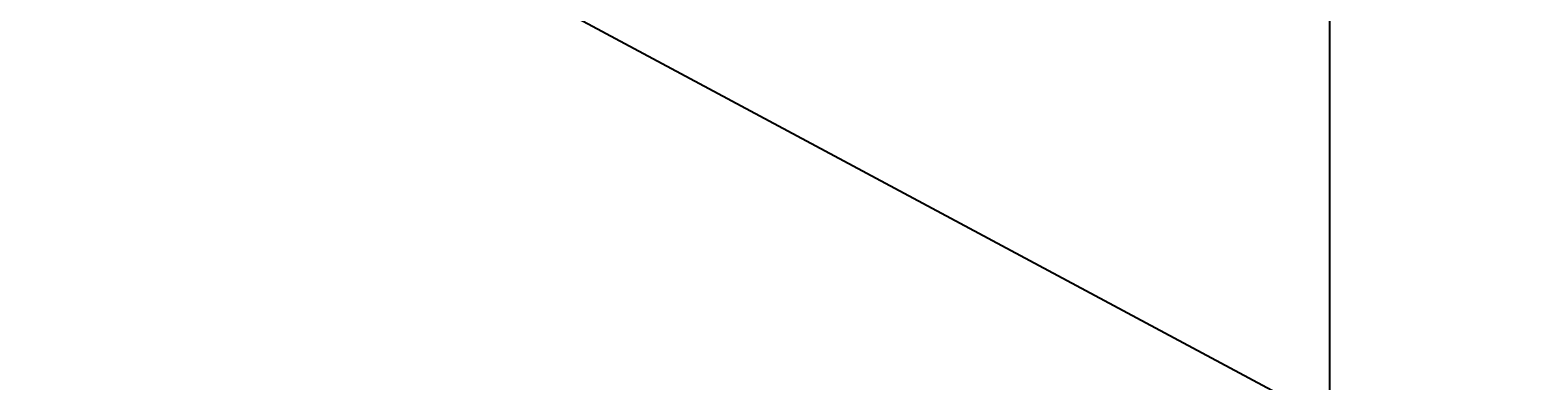
# Model space of a CAD drawing. Units: inches. Extents: x 35362 to 73946, y 43607 to 67532.
# Tile 118 of 134: x 50905 to 51049, y 49061 to 49095. Entities that reach past the tile are written whole.
import ezdxf

# ---------------------------------------------------------------- set-up
doc = ezdxf.new("R2010")
doc.units = ezdxf.units.IN
doc.header["$MEASUREMENT"] = 0
doc.layers.add('A-ANNO-DIMS', color=2, linetype='Continuous', lineweight=18)
doc.layers.add('E-SYMB', color=1, linetype='Continuous', lineweight=25)
doc.styles.get("Standard").update_dxf_attribs({"font": 'arial.ttf'})
doc.dimstyles.get("Standard").update_dxf_attribs({"dimtxt": 0.18, "dimasz": 0.18, "dimexe": 0.18, "dimexo": 0.0625, "dimgap": 0.09, "dimtad": 0, "dimtih": 1, "dimtoh": 1, "dimdec": 4, "dimzin": 0, "dimdsep": 46, "dimtxsty": 'Standard', "dimcen": 0.09, "dimadec": 0, "dimazin": 0, "dimtfac": 1, "dimtdec": 4, "dimtofl": 0, "dimtmove": 0, "dimatfit": 3, "dimfxl": 1, "dimtolj": 1, "dimtzin": 0, "dimarcsym": 0})

# ---------------------------------------------------------------- blocks, each defined once
blk = doc.blocks.new('*D11')
at = {"layer": 'A-ANNO-DIMS', "color": 0, "lineweight": -2, "transparency": 16777216}
for p, q in [((47978.66, 56028.77), (47978.66, 43606.68)), ((53109.76, 56028.77), (53109.76, 43606.68)), ((47978.84, 43606.86), (50543.87, 43606.86)), ((53109.58, 43606.86), (50544.55, 43606.86))]:
    blk.add_line(p, q, dxfattribs=at)
at = {"layer": 'A-ANNO-DIMS', "color": 0, "transparency": 16777216}
for points in [[(47978.84, 43606.89), (47978.84, 43606.83), (47978.66, 43606.86)], [(53109.58, 43606.89), (53109.58, 43606.83), (53109.76, 43606.86)]]:
    blk.add_solid(points, dxfattribs=at)
at = {"layer": 'Defpoints', "color": 0, "transparency": 16777216}
for p in [(47978.66, 56028.84), (53109.76, 56028.84), (53109.76, 43606.86)]:
    blk.add_point(p, dxfattribs=at)
at = {"layer": 'A-ANNO-DIMS', "color": 0, "transparency": 16777216, "insert": (50544.21, 43606.86), "char_height": 0.18, "attachment_point": 5}
blk.add_mtext('\\A1;5131', dxfattribs=at)
blk = doc.blocks.new('*D13')
at = {"layer": 'A-ANNO-DIMS', "color": 0, "lineweight": -2, "transparency": 16777216}
for p, q in [((48373.49, 51694.02), (48373.49, 43606.68)), ((51029.04, 51694.02), (51029.04, 43606.68)), ((48373.67, 43606.86), (49700.8, 43606.86)), ((51028.86, 43606.86), (49701.73, 43606.86))]:
    blk.add_line(p, q, dxfattribs=at)
at = {"layer": 'A-ANNO-DIMS', "color": 0, "transparency": 16777216}
for points in [[(48373.67, 43606.89), (48373.67, 43606.83), (48373.49, 43606.86)], [(51028.86, 43606.89), (51028.86, 43606.83), (51029.04, 43606.86)]]:
    blk.add_solid(points, dxfattribs=at)
at = {"layer": 'Defpoints', "color": 0, "transparency": 16777216}
for p in [(48373.49, 51694.09), (51029.04, 51694.09), (51029.04, 43606.86)]:
    blk.add_point(p, dxfattribs=at)
at = {"layer": 'A-ANNO-DIMS', "color": 0, "transparency": 16777216, "insert": (49701.27, 43606.86), "char_height": 0.18, "attachment_point": 5}
blk.add_mtext('\\A1;2655.6', dxfattribs=at)
blk = doc.blocks.new('*D17')
at = {"layer": 'A-ANNO-DIMS', "color": 0, "lineweight": -2, "transparency": 16777216}
for p, q in [((49923.31, 61293.22), (49923.31, 43606.68)), ((51913.93, 61293.22), (51913.93, 43606.68)), ((49923.49, 43606.86), (50918.16, 43606.86)), ((51913.75, 43606.86), (50919.07, 43606.86))]:
    blk.add_line(p, q, dxfattribs=at)
at = {"layer": 'A-ANNO-DIMS', "color": 0, "transparency": 16777216}
for points in [[(49923.49, 43606.89), (49923.49, 43606.83), (49923.31, 43606.86)], [(51913.75, 43606.89), (51913.75, 43606.83), (51913.93, 43606.86)]]:
    blk.add_solid(points, dxfattribs=at)
at = {"layer": 'Defpoints', "color": 0, "transparency": 16777216}
for p in [(49923.31, 61293.29), (51913.93, 61293.29), (51913.93, 43606.86)]:
    blk.add_point(p, dxfattribs=at)
at = {"layer": 'A-ANNO-DIMS', "color": 0, "transparency": 16777216, "insert": (50918.62, 43606.86), "char_height": 0.18, "attachment_point": 5}
blk.add_mtext('\\A1;1990.6', dxfattribs=at)
blk = doc.blocks.new('*D67')
at = {"layer": 'A-ANNO-DIMS', "color": 0, "lineweight": -2, "transparency": 16777216}
for p, q in [((56873.54, 53351.53), (35361.77, 53351.53)), ((35361.95, 53351.35), (35361.95, 49400.89)), ((35361.95, 45450.07), (35361.95, 49400.53)), ((53793.58, 45449.89), (35361.77, 45449.89))]:
    blk.add_line(p, q, dxfattribs=at)
at = {"layer": 'A-ANNO-DIMS', "color": 0, "transparency": 16777216}
for points in [[(35361.92, 53351.35), (35361.98, 53351.35), (35361.95, 53351.53)], [(35361.92, 45450.07), (35361.98, 45450.07), (35361.95, 45449.89)]]:
    blk.add_solid(points, dxfattribs=at)
at = {"layer": 'Defpoints', "color": 0, "transparency": 16777216}
for p in [(35361.95, 53351.53), (56873.6, 53351.53), (53793.64, 45449.89)]:
    blk.add_point(p, dxfattribs=at)
at = {"layer": 'A-ANNO-DIMS', "color": 0, "transparency": 16777216, "insert": (35361.95, 49400.71), "char_height": 0.18, "attachment_point": 5}
blk.add_mtext('\\A1;7901.6', dxfattribs=at)
blk = doc.blocks.new('*D84')
at = {"layer": 'A-ANNO-DIMS', "color": 0, "lineweight": -2, "transparency": 16777216}
for p, q in [((55540.23, 49259.94), (35361.77, 49259.94)), ((35361.95, 49259.76), (35361.95, 49115.14)), ((35361.95, 48970.16), (35361.95, 49114.78)), ((55540.23, 48969.98), (35361.77, 48969.98))]:
    blk.add_line(p, q, dxfattribs=at)
at = {"layer": 'A-ANNO-DIMS', "color": 0, "transparency": 16777216}
for points in [[(35361.92, 49259.76), (35361.98, 49259.76), (35361.95, 49259.94)], [(35361.92, 48970.16), (35361.98, 48970.16), (35361.95, 48969.98)]]:
    blk.add_solid(points, dxfattribs=at)
at = {"layer": 'Defpoints', "color": 0, "transparency": 16777216}
for p in [(35361.95, 49259.94), (55540.3, 49259.94), (55540.3, 48969.98)]:
    blk.add_point(p, dxfattribs=at)
at = {"layer": 'A-ANNO-DIMS', "color": 0, "transparency": 16777216, "insert": (35361.95, 49114.96), "char_height": 0.18, "attachment_point": 5}
blk.add_mtext('\\A1;289.96', dxfattribs=at)
blk = doc.blocks.new('*D86')
at = {"layer": 'A-ANNO-DIMS', "color": 0, "lineweight": -2, "transparency": 16777216}
for p, q in [((51285.53, 49320.08), (35361.77, 49320.08)), ((35361.95, 49319.9), (35361.95, 49120.26)), ((35361.95, 48920.26), (35361.95, 49119.9)), ((51285.53, 48920.08), (35361.77, 48920.08))]:
    blk.add_line(p, q, dxfattribs=at)
at = {"layer": 'A-ANNO-DIMS', "color": 0, "transparency": 16777216}
for points in [[(35361.92, 49319.9), (35361.98, 49319.9), (35361.95, 49320.08)], [(35361.92, 48920.26), (35361.98, 48920.26), (35361.95, 48920.08)]]:
    blk.add_solid(points, dxfattribs=at)
at = {"layer": 'Defpoints', "color": 0, "transparency": 16777216}
for p in [(35361.95, 49320.08), (51285.59, 49320.08), (51285.59, 48920.08)]:
    blk.add_point(p, dxfattribs=at)
at = {"layer": 'A-ANNO-DIMS', "color": 0, "transparency": 16777216, "insert": (35361.95, 49120.08), "char_height": 0.18, "attachment_point": 5}
blk.add_mtext('\\A1;400.0', dxfattribs=at)
blk = doc.blocks.new('*D107')
at = {"layer": 'A-ANNO-DIMS', "color": 0, "lineweight": -2, "transparency": 16777216}
for p, q in [((50139.56, 59850.01), (50139.56, 43606.68)), ((51320.81, 59850.01), (51320.81, 43606.68)), ((50139.74, 43606.86), (50729.73, 43606.86)), ((51320.63, 43606.86), (50730.64, 43606.86))]:
    blk.add_line(p, q, dxfattribs=at)
at = {"layer": 'A-ANNO-DIMS', "color": 0, "transparency": 16777216}
for points in [[(50139.74, 43606.89), (50139.74, 43606.83), (50139.56, 43606.86)], [(51320.63, 43606.89), (51320.63, 43606.83), (51320.81, 43606.86)]]:
    blk.add_solid(points, dxfattribs=at)
at = {"layer": 'Defpoints', "color": 0, "transparency": 16777216}
for p in [(50139.56, 59850.08), (51320.81, 59850.08), (51320.81, 43606.86)]:
    blk.add_point(p, dxfattribs=at)
at = {"layer": 'A-ANNO-DIMS', "color": 0, "transparency": 16777216, "insert": (50730.19, 43606.86), "char_height": 0.18, "attachment_point": 5}
blk.add_mtext('\\A1;1181.3', dxfattribs=at)

msp = doc.modelspace()

# ---------------------------------------------------------------- linework, layer by layer
at = {"layer": 'E-SYMB'}
msp.add_line((50952.662, 49098.368), (51285.595, 48920.079), dxfattribs=at)

# ---------------------------------------------------------------- dimensions: what is measured, and where the dimension line sits
at = {"layer": 'A-ANNO-DIMS'}
for base, p1, p2, override, picture, middle in [((51913.931, 43606.859), (49923.307, 61293.286), (51913.931, 61293.286), {"dimdec": 1, "dimlfac": 1, "dimrnd": 0, "dimzin": 0, "dimdsep": 46, "dimlunit": 2}, '*D17', (50918.619, 43606.859)), ((51320.8133, 43606.859), (50139.5627, 59850.0769), (51320.8133, 59850.0769), {"dimdec": 1, "dimlfac": 1, "dimrnd": 0, "dimzin": 0, "dimdsep": 46, "dimlunit": 2}, '*D107', (50730.188, 43606.859)), ((53109.76, 43606.859), (47978.665, 56028.836), (53109.76, 56028.836), {"dimdec": 0, "dimlfac": 1, "dimrnd": 0, "dimzin": 0, "dimdsep": 46, "dimlunit": 2}, '*D11', (50544.212, 43606.859)), ((51029.043, 43606.859), (48373.492, 51694.087), (51029.043, 51694.087), {"dimdec": 1, "dimlfac": 1, "dimrnd": 0, "dimzin": 0, "dimdsep": 46, "dimlunit": 2}, '*D13', (49701.267, 43606.859))]:
    dim = msp.add_linear_dim(base=base, p1=p1, p2=p2, dimstyle='Standard', override=override, dxfattribs=at)
    dim.commit()
    dim.dimension.update_dxf_attribs({"geometry": picture, "text_midpoint": middle})
for base, p1, p2, override, picture, middle in [((35361.949, 53351.529), (53793.638, 45449.894), (56873.602, 53351.529), {"dimdec": 1, "dimlfac": 1, "dimrnd": 0, "dimzin": 0, "dimdsep": 46, "dimlunit": 2}, '*D67', (35361.949, 49400.712)), ((35361.949, 49320.079), (51285.595, 48920.079), (51285.595, 49320.079), {"dimdec": 1, "dimlfac": 1, "dimrnd": 0, "dimzin": 0, "dimdsep": 46, "dimlunit": 2}, '*D86', (35361.949, 49120.079)), ((35361.9491, 49259.9353), (55540.2972, 48969.9796), (55540.2972, 49259.9353), {"dimdec": 2, "dimlfac": 1, "dimrnd": 0, "dimzin": 0, "dimdsep": 46, "dimlunit": 2}, '*D84', (35361.9491, 49114.9575))]:
    dim = msp.add_linear_dim(base=base, p1=p1, p2=p2, angle=90, dimstyle='Standard', override=override, dxfattribs=at)
    dim.commit()
    dim.dimension.update_dxf_attribs({"geometry": picture, "text_midpoint": middle})

doc.saveas('drawing.dxf')
